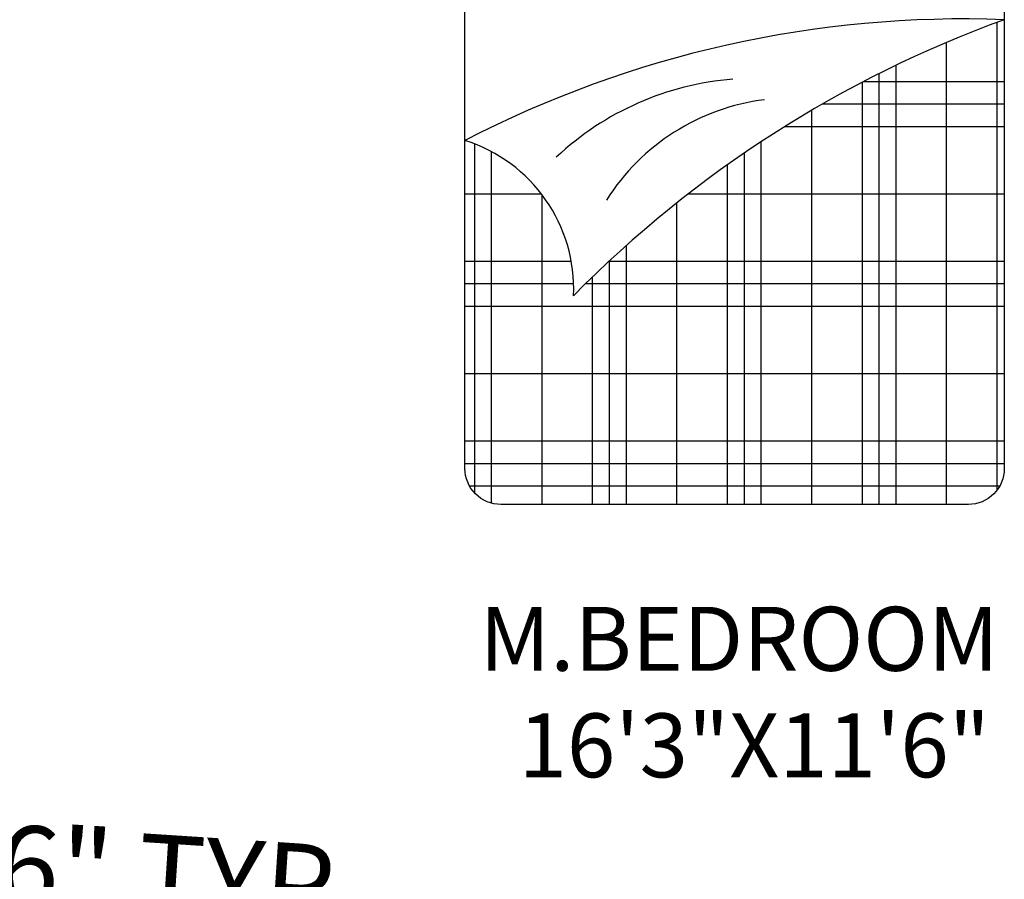
# Model space of a CAD drawing. Units: inches. Extents: x 3064 to 19385, y 846 to 15425.
# Tile 75 of 108: x 6629 to 6737, y 1870 to 1964. Entities that reach past the tile are written whole.
import ezdxf

# ---------------------------------------------------------------- set-up
doc = ezdxf.new("R2010")
doc.units = ezdxf.units.IN
for name, color, linetype, lineweight in [('A-ANNO-DIMS', 2, 'Continuous', 18), ('A-AREA-IDEN', 3, 'Continuous', 18), ('A-FLOR-FIXT', 9, 'Continuous', 18)]:
    doc.layers.add(name, color=color, linetype=linetype, lineweight=lineweight)
doc.layers.add('BLOCK', color=6, linetype='Continuous')
doc.styles.get("Standard").update_dxf_attribs({"font": 'arial.ttf'})
doc.dimstyles.new('ISO-25', dxfattribs={"dimtxt": 9, "dimasz": 2.5, "dimexe": 1.25, "dimexo": 0.625, "dimtad": 1, "dimdec": 1, "dimlunit": 3, "dimtxsty": 'Standard', "dimcen": 2.5, "dimadec": 0, "dimazin": 0, "dimtfac": 1, "dimtdec": 1, "dimtmove": 0, "dimatfit": 3, "dimfxl": 1, "dimarcsym": 0})

# ---------------------------------------------------------------- blocks, each defined once
blk = doc.blocks.new('*X5')
at = {"color": 0}
for p, q in [((276.598, 451.25), (280.51, 451.25)), ((275.455, 450.625), (280.51, 450.625)), ((274.411, 450), (280.51, 450)), ((265.51, 448.125), (267.634, 448.125)), ((271.723, 448.125), (280.51, 448.125)), ((265.51, 446.25), (268.465, 446.25)), ((269.519, 446.25), (280.51, 446.25)), ((265.51, 445.625), (268.531, 445.625)), ((268.866, 445.625), (280.51, 445.625)), ((265.51, 445), (280.51, 445)), ((265.51, 443.125), (280.51, 443.125)), ((265.51, 441.25), (280.51, 441.25)), ((265.51, 440.625), (280.51, 440.625)), ((265.634, 440), (280.386, 440))]:
    blk.add_line(p, q, dxfattribs=at)
blk = doc.blocks.new('*X6')
at = {"color": 0}
for p, q in [((280.312, 439.886), (280.312, 452.896)), ((278.906, 439.482), (278.906, 452.338)), ((277.5, 439.482), (277.5, 451.702)), ((277.031, 439.482), (277.031, 451.471)), ((276.562, 439.482), (276.562, 451.231)), ((275.156, 439.482), (275.156, 450.451)), ((265.781, 439.797), (265.781, 449.511)), ((273.75, 439.482), (273.75, 449.576)), ((266.25, 439.517), (266.25, 449.296)), ((273.281, 439.482), (273.281, 449.261)), ((272.812, 439.482), (272.812, 448.934)), ((267.656, 439.482), (267.656, 448.095)), ((271.406, 439.482), (271.406, 447.876)), ((270, 439.482), (270, 446.689)), ((269.531, 439.482), (269.531, 446.262)), ((269.062, 439.482), (269.062, 445.817))]:
    blk.add_line(p, q, dxfattribs=at)
blk = doc.blocks.new('A$C52E67D0D')
at = {"layer": 'BLOCK'}
blk.add_lwpolyline([(1901, 0), (601, 0, -0.414214), (501, 100), (501, 1700, -0.414214), (601, 1800), (1901, 1800, -0.414214), (2001, 1700), (2001, 100, -0.414214)], format="xyb", close=True, dxfattribs=at)
for centre, radius, start, end in [((1888.6, -1664.5), 3015.3, 87.8642, 117.4001), ((3101, -1685.8), 3227.7, 109.926, 135.3977), ((1308.8, 377.9), 807.6, 94.4436, 133.2788), ((1410.8, 520.2), 610.8, 97.2157, 147.6656), ((371.4, 600.4), 432, 357.3792, 72.5379)]:
    blk.add_arc(centre, radius, start, end, dxfattribs=at)
at = {"layer": 'BLOCK', "xscale": 100, "yscale": 100, "zscale": 100}
for name in ['*X6', '*X5']:
    blk.add_blockref(name, (-26050, -43948.2), dxfattribs=at)
blk = doc.blocks.new('*D433')
at = {"layer": 'A-ANNO-DIMS', "color": 0, "lineweight": -2, "transparency": 16777216}
for p, q in [((6621.84, 1945.07), (6633.12, 2118.25)), ((6612.14, 1945.71), (6623.09, 1944.99)), ((6617.52, 1878.71), (6621.68, 1942.58)), ((6607.65, 1876.85), (6618.61, 1876.14))]:
    blk.add_line(p, q, dxfattribs=at)
at = {"layer": 'A-ANNO-DIMS', "color": 0, "transparency": 16777216}
for points in [[(6621.26, 1942.61), (6622.09, 1942.55), (6621.84, 1945.07)], [(6617.11, 1878.74), (6617.94, 1878.69), (6617.36, 1876.22)]]:
    blk.add_solid(points, dxfattribs=at)
at = {"layer": 'Defpoints', "color": 0, "transparency": 16777216}
for p in [(6611.51, 1945.75), (6621.84, 1945.07), (6607.03, 1876.89)]:
    blk.add_point(p, dxfattribs=at)
at = {"layer": 'A-ANNO-DIMS', "color": 0, "transparency": 16777216, "insert": (6622.29, 2033.25), "char_height": 9, "attachment_point": 5, "rotation": 86.2748}
blk.add_mtext('WINDOW W1900-A 5\'-9" TYP.', dxfattribs=at)
blk = doc.blocks.new('*D434')
at = {"layer": 'A-ANNO-DIMS', "color": 0, "lineweight": -2, "transparency": 16777216}
for p, q in [((6601, 1876.66), (6600.29, 1865.71)), ((6606.99, 1876.27), (6606.28, 1865.32)), ((6597.88, 1867.12), (6595.38, 1867.28)), ((6600.37, 1866.95), (6606.36, 1866.56)), ((6608.85, 1866.4), (6667.34, 1862.59))]:
    blk.add_line(p, q, dxfattribs=at)
at = {"layer": 'A-ANNO-DIMS', "color": 0, "transparency": 16777216}
for points in [[(6597.9, 1867.53), (6597.85, 1866.7), (6600.37, 1866.95)], [(6608.88, 1866.82), (6608.83, 1865.99), (6606.36, 1866.56)]]:
    blk.add_solid(points, dxfattribs=at)
at = {"layer": 'Defpoints', "color": 0, "transparency": 16777216}
for p in [(6601.04, 1877.28), (6607.03, 1876.89), (6606.36, 1866.56)]:
    blk.add_point(p, dxfattribs=at)
at = {"layer": 'A-ANNO-DIMS', "color": 0, "transparency": 16777216, "insert": (6639.68, 1869.62), "char_height": 9, "attachment_point": 5, "rotation": 356.2748}
blk.add_mtext('0\'-6" TYP.', dxfattribs=at)

msp = doc.modelspace()

# ---------------------------------------------------------------- block references
at = {"layer": 'A-FLOR-FIXT', "xscale": 0.039370099999992, "yscale": 0.039370099999992, "zscale": 0.039370099999992}
msp.add_blockref('A$C52E67D0D', (6658.28, 1911.12), dxfattribs=at)

# ---------------------------------------------------------------- texts
at = {"layer": 'A-AREA-IDEN', "insert": (6679.59, 1899.9), "char_height": 7, "attachment_point": 1}
msp.add_mtext_dynamic_manual_height_columns('M.BEDROOM\\P  16\'3"X11\'6"', width=67.5924, gutter_width=12.5, heights=[0], dxfattribs=at)

# ---------------------------------------------------------------- dimensions: what is measured, and where the dimension line sits
at = {"layer": 'A-ANNO-DIMS'}
for base, p1, p2, angle, text, picture, middle in [((6621.84, 1945.07), (6607.03, 1876.89), (6611.51, 1945.75), 86.2748, 'WINDOW W1900-A <> TYP.', '*D433', (6622.29, 2033.25)), ((6606.36, 1866.56), (6601.04, 1877.28), (6607.03, 1876.89), 356.2748, '<> TYP.', '*D434', (6639.68, 1869.62))]:
    dim = msp.add_linear_dim(base=base, p1=p1, p2=p2, angle=angle, text=text, dimstyle='ISO-25', override={"dimdec": 1, "dimrnd": 0, "dimzin": 1, "dimlunit": 4, "dimfrac": 2}, dxfattribs=at)
    dim.commit()
    dim.dimension.update_dxf_attribs({"geometry": picture, "text_midpoint": middle})

doc.saveas('drawing.dxf')
